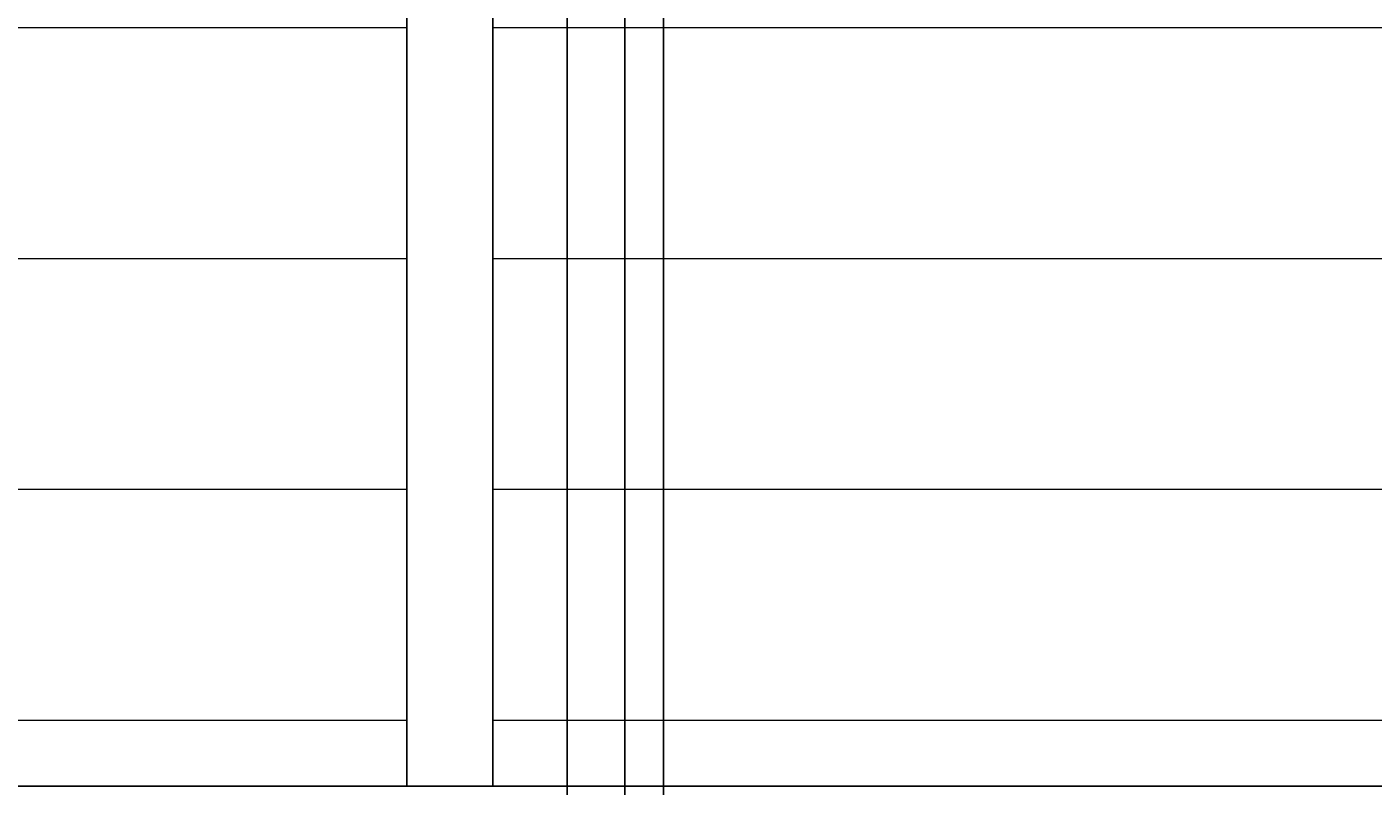
# Model space of a CAD drawing. Units: inches. Extents: x -6 to 289, y -8 to 323.
# Tile 29 of 107: x 174 to 209, y 10 to 30. Entities that reach past the tile are written whole.
import ezdxf

# ---------------------------------------------------------------- set-up
doc = ezdxf.new("R2010")
doc.units = ezdxf.units.IN
doc.header["$MEASUREMENT"] = 0
for name, color, linetype, lineweight in [('A-ANNO-DIMS', 2, 'Continuous', 18), ('A-DOOR', 3, 'Continuous', 25), ('A-ELEV-PATT', 8, 'Continuous', 13)]:
    doc.layers.add(name, color=color, linetype=linetype, lineweight=lineweight)
doc.styles.get("Standard").update_dxf_attribs({"font": 'arial.ttf'})
doc.dimstyles.get("Standard").update_dxf_attribs({"dimtxt": 0.18, "dimasz": 0.18, "dimexe": 0.18, "dimexo": 0.0625, "dimgap": 0.09, "dimtad": 0, "dimtih": 1, "dimtoh": 1, "dimdec": 4, "dimzin": 0, "dimdsep": 46, "dimtxsty": 'Standard', "dimcen": 0.09, "dimadec": 0, "dimazin": 0, "dimtfac": 1, "dimtdec": 4, "dimtofl": 0, "dimtmove": 0, "dimatfit": 3, "dimfxl": 1, "dimtolj": 1, "dimtzin": 0, "dimarcsym": 0})

# ---------------------------------------------------------------- blocks, each defined once
blk = doc.blocks.new('*D16')
at = {"layer": 'A-ANNO-DIMS', "color": 0, "lineweight": -2, "transparency": 16777216}
for p, q in [((9.943, 68.37), (9.943, -8.391)), ((272.973, 68.37), (272.973, -8.391)), ((10.123, -8.211), (140.993, -8.211)), ((272.793, -8.211), (141.923, -8.211))]:
    blk.add_line(p, q, dxfattribs=at)
at = {"layer": 'A-ANNO-DIMS', "color": 0, "transparency": 16777216}
for points in [[(10.123, -8.181), (10.123, -8.241), (9.943, -8.211)], [(272.793, -8.181), (272.793, -8.241), (272.973, -8.211)]]:
    blk.add_solid(points, dxfattribs=at)
at = {"layer": 'Defpoints', "color": 0, "transparency": 16777216}
for p in [(9.943, 68.432), (272.973, 68.432), (272.973, -8.211)]:
    blk.add_point(p, dxfattribs=at)
at = {"layer": 'A-ANNO-DIMS', "color": 0, "transparency": 16777216, "insert": (141.458, -8.211), "char_height": 0.18, "attachment_point": 5}
blk.add_mtext('\\A1;263.03', dxfattribs=at)
blk = doc.blocks.new('*D40')
at = {"layer": 'A-ANNO-DIMS', "color": 0, "lineweight": -2, "transparency": 16777216}
for p, q in [((188.292, 226.826), (188.292, -8.391)), ((189.792, 225.326), (189.792, -8.391)), ((188.472, -8.211), (188.796, -8.211)), ((189.612, -8.211), (189.288, -8.211))]:
    blk.add_line(p, q, dxfattribs=at)
at = {"layer": 'A-ANNO-DIMS', "color": 0, "transparency": 16777216}
for points in [[(188.472, -8.181), (188.472, -8.241), (188.292, -8.211)], [(189.612, -8.181), (189.612, -8.241), (189.792, -8.211)]]:
    blk.add_solid(points, dxfattribs=at)
at = {"layer": 'Defpoints', "color": 0, "transparency": 16777216}
for p in [(188.292, 226.889), (189.792, 225.389), (189.792, -8.211)]:
    blk.add_point(p, dxfattribs=at)
at = {"layer": 'A-ANNO-DIMS', "color": 0, "transparency": 16777216, "insert": (189.042, -8.211), "char_height": 0.18, "attachment_point": 5}
blk.add_mtext('\\A1;1.5', dxfattribs=at)
blk = doc.blocks.new('*D41')
at = {"layer": 'A-ANNO-DIMS', "color": 0, "lineweight": -2, "transparency": 16777216}
for p, q in [((189.792, 225.326), (189.792, -8.391)), ((190.792, 224.326), (190.792, -8.391)), ((189.972, -8.211), (190.169, -8.211)), ((190.612, -8.211), (190.415, -8.211))]:
    blk.add_line(p, q, dxfattribs=at)
at = {"layer": 'A-ANNO-DIMS', "color": 0, "transparency": 16777216}
for points in [[(189.972, -8.181), (189.972, -8.241), (189.792, -8.211)], [(190.612, -8.181), (190.612, -8.241), (190.792, -8.211)]]:
    blk.add_solid(points, dxfattribs=at)
at = {"layer": 'Defpoints', "color": 0, "transparency": 16777216}
for p in [(189.792, 225.389), (190.792, 224.389), (190.792, -8.211)]:
    blk.add_point(p, dxfattribs=at)
at = {"layer": 'A-ANNO-DIMS', "color": 0, "transparency": 16777216, "insert": (190.292, -8.211), "char_height": 0.18, "attachment_point": 5}
blk.add_mtext('\\A1;1', dxfattribs=at)
blk = doc.blocks.new('*D42')
at = {"layer": 'A-ANNO-DIMS', "color": 0, "lineweight": -2, "transparency": 16777216}
for p, q in [((190.792, 224.326), (190.792, -8.391)), ((211.292, 224.326), (211.292, -8.391)), ((190.972, -8.211), (200.716, -8.211)), ((211.112, -8.211), (201.368, -8.211))]:
    blk.add_line(p, q, dxfattribs=at)
at = {"layer": 'A-ANNO-DIMS', "color": 0, "transparency": 16777216}
for points in [[(190.972, -8.181), (190.972, -8.241), (190.792, -8.211)], [(211.112, -8.181), (211.112, -8.241), (211.292, -8.211)]]:
    blk.add_solid(points, dxfattribs=at)
at = {"layer": 'Defpoints', "color": 0, "transparency": 16777216}
for p in [(190.792, 224.389), (211.292, 224.389), (211.292, -8.211)]:
    blk.add_point(p, dxfattribs=at)
at = {"layer": 'A-ANNO-DIMS', "color": 0, "transparency": 16777216, "insert": (201.042, -8.211), "char_height": 0.18, "attachment_point": 5}
blk.add_mtext('\\A1;20.5', dxfattribs=at)

msp = doc.modelspace()

# ---------------------------------------------------------------- hatches: boundary and pattern name
at = {"layer": 'A-ELEV-PATT'}
h = msp.add_hatch(dxfattribs=at)
h.set_pattern_fill('_USER', color=256, scale=6, pattern_type=0)
h.set_pattern_definition([(0, (0, 0), (0, 6), [])])
h.paths.add_polyline_path([(184.1244, 48.0851), (124.008, 48.0851), (124.008, 10.2888), (184.1244, 10.2888)])
h.paths.add_polyline_path([(244.2408, 48.0851), (186.3604, 48.0851), (186.3604, 10.2888), (244.2408, 10.2888)])
h.paths.add_polyline_path([(208.2918, 114.2795), (190.7918, 114.2795), (190.7918, 71.2795), (208.2918, 71.2795)])
h.paths.add_polyline_path([(227.7918, 114.2795), (209.2918, 114.2795), (209.2918, 71.2795), (227.7918, 71.2795)])
h.paths.add_polyline_path([(211.2918, 224.3887), (190.7918, 224.3887), (190.7918, 162.3484), (211.2918, 162.3484)])
h.paths.add_polyline_path([(233.7918, 224.3887), (212.2918, 224.3887), (212.2918, 162.3484), (233.7918, 162.3484)])
h.paths.add_polyline_path([(166.3835, 224.154), (147.8835, 224.154), (147.8835, 181.154), (166.3835, 181.154)])
h.paths.add_polyline_path([(146.8835, 224.154), (129.3835, 224.154), (129.3835, 181.154), (146.8835, 181.154)])

# ---------------------------------------------------------------- linework, layer by layer
at = {"layer": 'A-DOOR'}
for points in [[(124.008, 48.0851), (244.2408, 48.0851), (244.2408, 10.2888), (124.008, 10.2888)], [(184.1244, 48.0851), (186.3604, 48.0851), (186.3604, 10.2888), (184.1244, 10.2888)]]:
    msp.add_lwpolyline(points, close=True, dxfattribs=at)

# ---------------------------------------------------------------- dimensions: what is measured, and where the dimension line sits
at = {"layer": 'A-ANNO-DIMS'}
for base, p1, p2, override, picture, middle in [((189.7918, -8.2112), (188.2918, 226.8887), (189.7918, 225.3887), {"dimdec": 1, "dimlfac": 1, "dimrnd": 0, "dimzin": 0, "dimdsep": 46, "dimlunit": 2}, '*D40', (189.0418, -8.2112)), ((190.7918, -8.2112), (189.7918, 225.3887), (190.7918, 224.3887), {"dimdec": 0, "dimlfac": 1, "dimrnd": 0, "dimzin": 0, "dimdsep": 46, "dimlunit": 2}, '*D41', (190.2918, -8.2112)), ((211.2918, -8.2112), (190.7918, 224.3887), (211.2918, 224.3887), {"dimdec": 1, "dimlfac": 1, "dimrnd": 0, "dimzin": 0, "dimdsep": 46, "dimlunit": 2}, '*D42', (201.0418, -8.2112)), ((272.9733, -8.2112), (9.943, 68.4322), (272.9733, 68.4322), {"dimdec": 2, "dimlfac": 1, "dimrnd": 0, "dimzin": 0, "dimdsep": 46, "dimlunit": 2}, '*D16', (141.4581, -8.2112))]:
    dim = msp.add_linear_dim(base=base, p1=p1, p2=p2, dimstyle='Standard', override=override, dxfattribs=at)
    dim.commit()
    dim.dimension.update_dxf_attribs({"geometry": picture, "text_midpoint": middle})

doc.saveas('drawing.dxf')
